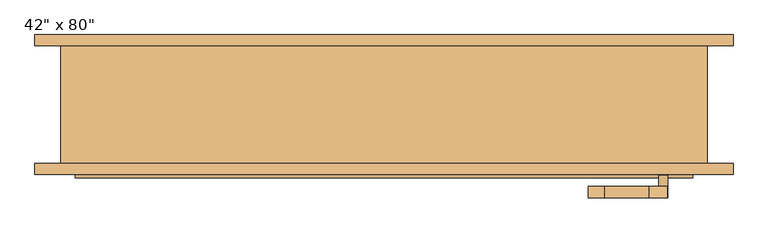
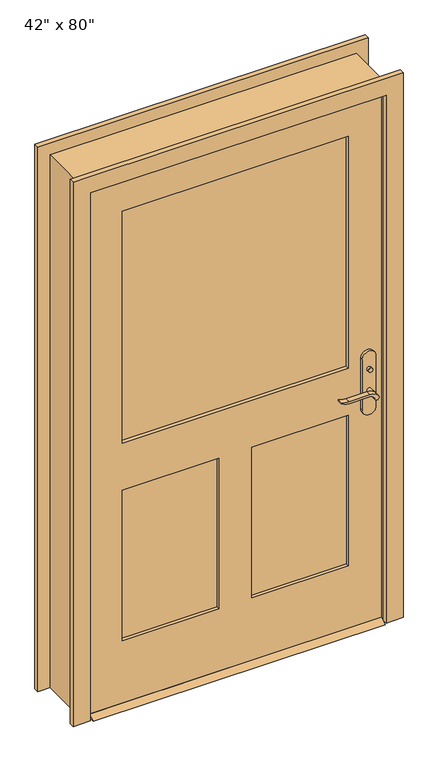
"""IFC4 building model written with IfcOpenShell, lengths in millimetres: door geometry."""

from ifc_helpers import new_model, si_unit, point, frame, frame_2d, origin, place, context, project, spatial, polyline, circle_curve, trimmed, segment, composite_curve, outline, extrude, faceted_brep, source, transform, mapped, element, save


def door_374e07cf(model_context):
    return source(origin(), model_context, "Body", "SolidModel", [
        extrude(outline(polyline([(-63.5, 12.7), (-38.1, 0.0), (-123.825, 0.0), (-98.425, 12.7), (-63.5, 12.7)])), frame((-533.4, 0.0, 0.0), z_axis=(1.0, 0.0, 0.0), x_axis=(0.0, 1.0, 0.0)), (0.0, 0.0, 1.0), 1066.8),
        extrude(outline(polyline([(487.6, -43.5), (487.6, -53.5), (477.6, -53.5), (477.6, -43.5), (487.6, -43.5)])), frame((0.0, 0.0, 981.9), z_axis=(0.0, 0.0, 1.0), x_axis=(1.0, 0.0, 0.0)), (0.0, 0.0, 1.0), 30.0),
        extrude(outline(composite_curve([segment(trimmed(circle_curve(frame_2d((996.9, 482.6)), 8.0), [point((996.9, 474.6))], [point((996.9, 490.6))], False, "CARTESIAN"), True, "CONTINUOUS"), segment(trimmed(circle_curve(frame_2d((996.9, 482.6)), 8.0), [point((996.9, 490.6))], [point((996.9, 474.6))], False, "CARTESIAN"), True, "CONTINUOUS")], self_intersect=False)), frame((0.0, -118.425, 0.0), z_axis=(0.0, 1.0, 0.0), x_axis=(0.0, 0.0, 1.0)), (0.0, 0.0, 1.0), 10.0),
        extrude(outline(composite_curve([segment(trimmed(circle_curve(frame_2d((897.1555521, 458.9324871)), 37.2832219), [point((919.0523287, 489.1081363))], [point((934.4, 457.2325667))], False, "CARTESIAN"), True, "CONTINUOUS"), segment(polyline([(934.4, 457.2325667), (934.4, 380.9564091)]), True, "CONTINUOUS"), segment(trimmed(circle_curve(frame_2d((1017.6850638, 381.0227909)), 83.2850902), [point((934.4, 380.9564091))], [point((939.4, 352.6))], True, "CARTESIAN"), True, "CONTINUOUS"), segment(polyline([(939.4, 352.6), (936.6135558, 352.6)]), True, "CONTINUOUS"), segment(trimmed(circle_curve(frame_2d((986.6709207, 384.5396612)), 59.3791355), [point((936.6135558, 352.6))], [point((927.4, 380.9564091))], False, "CARTESIAN"), True, "CONTINUOUS"), segment(polyline([(927.4, 380.9564091), (927.4, 457.2138099)]), True, "CONTINUOUS"), segment(trimmed(circle_curve(frame_2d((909.2738613, 457.2138099)), 18.1261387), [point((927.4, 457.2138099))], [point((914.4, 474.6))], True, "CARTESIAN"), True, "CONTINUOUS"), segment(trimmed(circle_curve(frame_2d((914.4, 482.6)), 8.0), [point((914.4, 474.6))], [point((919.0523287, 489.1081363))], False, "CARTESIAN"), True, "CONTINUOUS")], self_intersect=False)), frame((0.0, -23.5, 0.0), z_axis=(0.0, 1.0, 0.0), x_axis=(0.0, 0.0, 1.0)), (0.0, 0.0, 1.0), 20.0),
        extrude(outline(composite_curve([segment(trimmed(circle_curve(frame_2d((914.4, 482.6)), 8.0), [point((914.3999903, 474.6))], [point((919.0523287, 489.1081363))], False, "CARTESIAN"), True, "CONTINUOUS"), segment(trimmed(circle_curve(frame_2d((897.1555521, 458.9324871)), 37.2832219), [point((919.0523287, 489.1081363))], [point((934.4, 457.2325667))], False, "CARTESIAN"), True, "CONTINUOUS"), segment(polyline([(934.4, 457.2325667), (934.4, 380.9564091)]), True, "CONTINUOUS"), segment(trimmed(circle_curve(frame_2d((1017.6850638, 381.0227909)), 83.2850902), [point((934.4, 380.9564091))], [point((939.4, 352.6))], True, "CARTESIAN"), True, "CONTINUOUS"), segment(polyline([(939.4, 352.6), (936.6135558, 352.6)]), True, "CONTINUOUS"), segment(trimmed(circle_curve(frame_2d((986.6709207, 384.5396612)), 59.3791355), [point((936.6135558, 352.6))], [point((927.4, 380.9564091))], False, "CARTESIAN"), True, "CONTINUOUS"), segment(polyline([(927.4, 380.9564091), (927.4, 457.2138122)]), True, "CONTINUOUS"), segment(trimmed(circle_curve(frame_2d((909.2738682, 457.2138122)), 18.1261318), [point((927.4, 457.2138122))], [point((914.3999903, 474.6))], True, "CARTESIAN"), True, "CONTINUOUS")], self_intersect=False)), frame((0.0, -158.425, 0.0), z_axis=(0.0, 1.0, 0.0), x_axis=(0.0, 0.0, 1.0)), (0.0, 0.0, 1.0), 20.0),
        extrude(outline(composite_curve([segment(trimmed(circle_curve(frame_2d((914.4, 482.6)), 8.0), [point((914.4, 474.6))], [point((914.4, 490.6))], False, "CARTESIAN"), True, "CONTINUOUS"), segment(trimmed(circle_curve(frame_2d((914.4, 482.6)), 8.0), [point((914.4, 490.6))], [point((914.4, 474.6))], False, "CARTESIAN"), True, "CONTINUOUS")], self_intersect=False)), frame((0.0, -53.5, 0.0), z_axis=(0.0, 1.0, 0.0), x_axis=(0.0, 0.0, 1.0)), (0.0, 0.0, 1.0), 30.0),
        extrude(outline(composite_curve([segment(trimmed(circle_curve(frame_2d((914.4, 482.6)), 8.0), [point((914.4, 474.6))], [point((914.4, 490.6))], False, "CARTESIAN"), True, "CONTINUOUS"), segment(trimmed(circle_curve(frame_2d((914.4, 482.6)), 8.0), [point((914.4, 490.6))], [point((914.4, 474.6))], False, "CARTESIAN"), True, "CONTINUOUS")], self_intersect=False)), frame((0.0, -138.425, 0.0), z_axis=(0.0, 1.0, 0.0), x_axis=(0.0, 0.0, 1.0)), (0.0, 0.0, 1.0), 30.0),
        extrude(outline(composite_curve([segment(polyline([(844.4, 507.6), (1039.4, 507.6)]), True, "CONTINUOUS"), segment(trimmed(circle_curve(frame_2d((1039.4, 482.6)), 25.0), [point((1039.4, 507.6))], [point((1039.4, 457.6))], False, "CARTESIAN"), True, "CONTINUOUS"), segment(polyline([(1039.4, 457.6), (844.4, 457.6)]), True, "CONTINUOUS"), segment(trimmed(circle_curve(frame_2d((844.4, 482.6)), 25.0), [point((844.4, 457.6))], [point((844.4, 507.6))], False, "CARTESIAN"), True, "CONTINUOUS")], self_intersect=False)), frame((0.0, -63.5, 0.0), z_axis=(0.0, 1.0, 0.0), x_axis=(0.0, 0.0, 1.0)), (0.0, 0.0, 1.0), 10.0),
        extrude(outline(composite_curve([segment(polyline([(844.4, 507.6), (1039.4, 507.6)]), True, "CONTINUOUS"), segment(trimmed(circle_curve(frame_2d((1039.4, 482.6)), 25.0), [point((1039.4, 507.6))], [point((1039.4, 457.6))], False, "CARTESIAN"), True, "CONTINUOUS"), segment(polyline([(1039.4, 457.6), (844.4, 457.6)]), True, "CONTINUOUS"), segment(trimmed(circle_curve(frame_2d((844.4, 482.6)), 25.0), [point((844.4, 457.6))], [point((844.4, 507.6))], False, "CARTESIAN"), True, "CONTINUOUS")], self_intersect=False)), frame((0.0, -108.425, 0.0), z_axis=(0.0, 1.0, 0.0), x_axis=(0.0, 0.0, 1.0)), (0.0, 0.0, 1.0), 10.0),
        extrude(outline(polyline([(2032.0, -533.4), (12.7, -533.4), (12.7, 533.4), (2032.0, 533.4), (2032.0, -533.4)]), holes=[polyline([(1016.0, -412.75), (1911.35, -412.75), (1911.35, 412.75), (1016.0, 412.75), (1016.0, -412.75)]), polyline([(835.025, -60.325), (254.0, -60.325), (254.0, -412.75), (835.025, -412.75), (835.025, -60.325)]), polyline([(835.025, 412.75), (254.0, 412.75), (254.0, 60.325), (835.025, 60.325), (835.025, 412.75)])]), frame((0.0, -98.425, 0.0), z_axis=(0.0, 1.0, 0.0), x_axis=(0.0, 0.0, 1.0)), (0.0, 0.0, 1.0), 34.925),
        faceted_brep([(558.8, -98.425, 0.0), (533.4, -98.425, 0.0), (533.4, -63.5, 0.0), (520.7, -63.5, 0.0), (520.7, -28.575, 0.0), (533.4, -28.575, 0.0), (533.4, 104.775, 0.0), (558.8, 104.775, 0.0), (558.8, 104.775, 2057.4), (558.8, -98.425, 2057.4), (533.4, 104.775, 2032.0), (-533.4, 104.775, 2032.0), (-533.4, 104.775, 0.0), (-558.8, 104.775, 0.0), (-558.8, 104.775, 2057.4), (533.4, -28.575, 2032.0), (520.7, -28.575, 2019.3), (-520.7, -28.575, 2019.3), (-520.7, -28.575, 0.0), (-533.4, -28.575, 0.0), (-533.4, -28.575, 2032.0), (520.7, -63.5, 2019.3), (533.4, -63.5, 2032.0), (-533.4, -63.5, 2032.0), (-533.4, -63.5, 0.0), (-520.7, -63.5, 0.0), (-520.7, -63.5, 2019.3), (533.4, -98.425, 2032.0), (-558.8, -98.425, 2057.4), (-558.8, -98.425, 0.0), (-533.4, -98.425, 0.0), (-533.4, -98.425, 2032.0)], [[[0, 1, 2, 3, 4, 5, 6, 7]], [[7, 8, 9, 0]], [[6, 10, 11, 12, 13, 14, 8, 7]], [[5, 15, 10, 6]], [[4, 16, 17, 18, 19, 20, 15, 5]], [[3, 21, 16, 4]], [[2, 22, 23, 24, 25, 26, 21, 3]], [[1, 27, 22, 2]], [[0, 9, 28, 29, 30, 31, 27, 1]], [[8, 14, 28, 9]], [[15, 20, 11, 10]], [[21, 26, 17, 16]], [[27, 31, 23, 22]], [[29, 13, 12, 19, 18, 25, 24, 30]], [[14, 13, 29, 28]], [[20, 19, 12, 11]], [[26, 25, 18, 17]], [[31, 30, 24, 23]]]),
        extrude(outline(polyline([(-60.325, -75.1416667), (-60.325, -86.7833333), (-412.75, -86.7833333), (-412.75, -75.1416667), (-60.325, -75.1416667)])), frame((0.0, 0.0, 254.0), z_axis=(0.0, 0.0, 1.0), x_axis=(1.0, 0.0, 0.0)), (0.0, 0.0, 1.0), 581.025),
        extrude(outline(polyline([(412.75, -75.1416667), (412.75, -86.7833333), (60.325, -86.7833333), (60.325, -75.1416667), (412.75, -75.1416667)])), frame((0.0, 0.0, 254.0), z_axis=(0.0, 0.0, 1.0), x_axis=(1.0, 0.0, 0.0)), (0.0, 0.0, 1.0), 581.025),
        extrude(outline(polyline([(412.75, -77.47), (412.75, -84.455), (-412.75, -84.455), (-412.75, -77.47), (412.75, -77.47)])), frame((0.0, 0.0, 1016.0), z_axis=(0.0, 0.0, 1.0), x_axis=(1.0, 0.0, 0.0)), (0.0, 0.0, 1.0), 895.35),
        extrude(outline(polyline([(0.0, -539.75), (2038.35, -539.75), (2038.35, 539.75), (0.0, 539.75), (0.0, 603.25), (2101.85, 603.25), (2101.85, -603.25), (0.0, -603.25), (0.0, -539.75)])), frame((0.0, 104.775, 0.0), z_axis=(0.0, 1.0, 0.0), x_axis=(0.0, 0.0, 1.0)), (0.0, 0.0, 1.0), 19.05),
        extrude(outline(polyline([(0.0, -539.75), (2038.35, -539.75), (2038.35, 539.75), (0.0, 539.75), (0.0, 603.25), (2101.85, 603.25), (2101.85, -603.25), (0.0, -603.25), (0.0, -539.75)])), frame((0.0, -117.475, 0.0), z_axis=(0.0, 1.0, 0.0), x_axis=(0.0, 0.0, 1.0)), (0.0, 0.0, 1.0), 19.05),
    ])


if __name__ == "__main__":
    model = new_model("IFC4")
    model_context = context("Model", 3, world=origin())
    ifc_project = project(units=[si_unit("LENGTHUNIT", "METRE", prefix="MILLI")], contexts=[model_context])
    site = spatial("IfcSite", under=ifc_project)
    building = spatial("IfcBuilding", under=site)
    placement = place(None, origin())
    door_shape = door_374e07cf(model_context)
    element("IfcDoor", 1, ObjectType="42\" x 80\"", at=placement, inside=building, context=model_context, shape_type="MappedRepresentation", body=[
        mapped(door_shape, transform((0.0, 0.0, 0.0), x_axis=(1.0, 0.0, 0.0), y_axis=(0.0, 1.0, 0.0), z_axis=(0.0, 0.0, 1.0))),
    ])
    save(model, "model.ifc")

# Revit data of these elements
# Type "42\" x 80\""
#   Type Mark = "9"
#   Assembly Code = "B2030100"
#   Analytic Construction = "French door, wood frame with single glass"
#   Top Rail = 0' - 4 3/4"
#   Threshold Offset [instance default] = 0' - 0 1/2"
#   Thickness = 0' - 1 3/8"
#   Thermal Resistance (R) = 1.0696 (h·ft²·°F)/BTU
#   Swing Angle [instance default] = 90.00°
#   Stiles = 0' - 4 3/4"
#   Rough Width = 3' - 8"
#   Rough Height = 6' - 9"
#   Lock Rail = 0' - 7 1/8"
#   Height = 6' - 8"
#   Width = 3' - 6"
#   Heat Transfer Coefficient (U) = 0.9350 BTU/(h·ft²·°F)
#   Door Offset [instance default] = 0' - 0"
#   Bottom Rail = 0' - 9 1/2"
#   Threshold [instance default] = yes
#   Function = 1
#   Exterior Trim [instance default] = yes
#   Trim Material = Cherry
#   Threshold Material = Cherry
#   Panel Material = Cherry
#   Glazing = Glass
#   Frame Material = Cherry
#   Door Handle Material = Aluminum
#   Visual Light Transmittance = 0
#   Solar Heat Gain Coefficient = 0
#   Wall Closure = (empty or 0)
#   Construction Type = (empty or 0)
# Element 1 (IfcDoor, "42\" x 80\"")
#   Materials on its faces: "Cherry", "Aluminum", "Glass"
# Materials
#   "Cherry": class "Wood", colour RGB 226 177 128, transparency 0, Description = "Prunus Serotina", Cost = 0
#   "Glass": class "Glass", colour RGB 0 128 192, transparency 0.75, Description = "Soda Lime Glass", Cost = 0
#   "Aluminum": class "Metal", colour RGB 247 247 247, transparency 0, Description = "Aluminum 6061", Cost = 0
